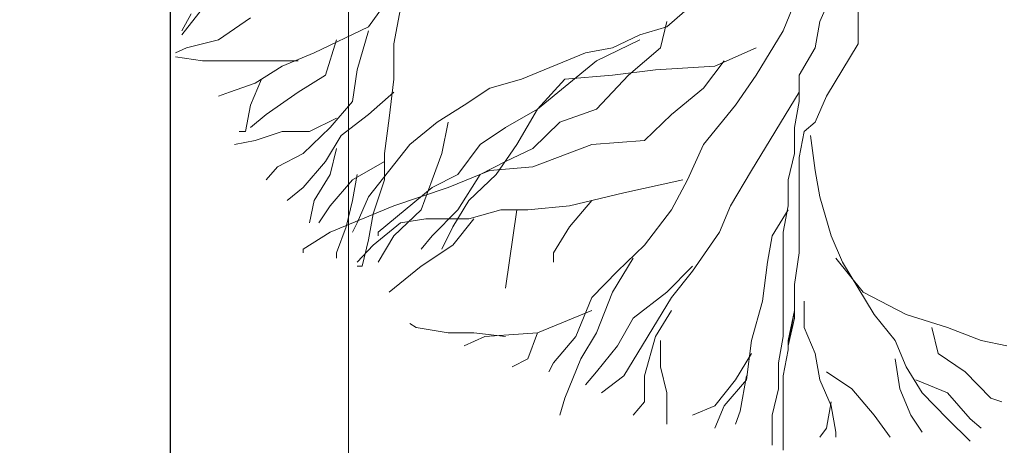
# Model space of a CAD drawing. Units: millimetres. Extents: x 595116 to 630915, y 909473 to 920225.
# Tile 15 of 134: x 629500 to 629534, y 919202 to 919216. Entities that reach past the tile are written whole.
import ezdxf

# ---------------------------------------------------------------- set-up
doc = ezdxf.new("R2010")
doc.units = ezdxf.units.MM
doc.layers.add('Dimension', color=3, linetype='Continuous', lineweight=18)
doc.layers.add('L-PLNT', color=85, linetype='Continuous', lineweight=13)
doc.styles.get("Standard").update_dxf_attribs({"font": 'arial.ttf'})
doc.dimstyles.new('ISO-25', dxfattribs={"dimtxt": 9, "dimasz": 6, "dimexe": 1.25, "dimexo": 0.625, "dimtad": 1, "dimlunit": 4, "dimtxsty": 'Standard', "dimcen": 2.5, "dimadec": 0, "dimazin": 0, "dimtfac": 1, "dimtmove": 0, "dimatfit": 3, "dimfxl": 1, "dimarcsym": 0})

# ---------------------------------------------------------------- blocks, each defined once
blk = doc.blocks.new('A$C143125F4')
for p, q in [((2.593, 1.7651), (2.593, 1.3932)), ((1.0011, 1.5724), (0.9136, 1.4515)), ((2.3906, 1.5724), (2.3359, 1.438)), ((2.4617, 1.4694), (2.5, 1.559)), ((2.0241, 1.5276), (1.9366, 1.4515)), ((0.2735, 1.4246), (0.3446, 1.5142)), ((0.3063, 1.4963), (0.2735, 1.438)), ((1.023, 1.5142), (1.0011, 1.3932)), ((0.5088, 1.4828), (0.3993, 1.4067)), ((1.9366, 1.4694), (1.9147, 1.3798)), ((2.4453, 1.3798), (2.4617, 1.4694)), ((0.9136, 1.4515), (0.7276, 1.3619)), ((0.9136, 1.438), (0.8753, 1.3036)), ((1.8436, 1.4246), (1.7506, 1.3798)), ((1.9366, 1.4515), (1.8436, 1.4246)), ((2.3359, 1.438), (2.2429, 1.2857)), ((0.3993, 1.4067), (0.2899, 1.3798)), ((0.8042, 1.4067), (0.7659, 1.2857)), ((1.0011, 1.3932), (1.0011, 1.2723)), ((1.8436, 1.4067), (1.6959, 1.335)), ((2.593, 1.3932), (2.4836, 1.214)), ((0.2899, 1.3798), (0.2516, 1.3619)), ((0.7276, 1.3619), (0.6182, 1.3171)), ((1.6576, 1.3619), (1.4387, 1.2723)), ((1.7506, 1.3798), (1.6576, 1.3619)), ((1.9147, 1.3798), (1.8053, 1.2857)), ((2.2429, 1.3798), (2.1007, 1.3171)), ((2.3906, 1.2857), (2.4453, 1.3798)), ((0.3446, 1.335), (0.2516, 1.3484)), ((0.6729, 1.335), (0.3446, 1.335)), ((0.6182, 1.3171), (0.5252, 1.2588)), ((1.6959, 1.335), (1.4935, 1.1692)), ((2.1007, 1.3171), (1.8983, 1.3036)), ((2.1335, 1.335), (2.0624, 1.2409)), ((0.7659, 1.2857), (0.6729, 1.2275)), ((0.8753, 1.3036), (0.8589, 1.1961)), ((1.7506, 1.2857), (1.5865, 1.2723)), ((1.8053, 1.2857), (1.6959, 1.1692)), ((1.8983, 1.3036), (1.7506, 1.2857)), ((2.2429, 1.2857), (2.1718, 1.1827)), ((2.3906, 1.1961), (2.3906, 1.2857)), ((0.5252, 1.2588), (0.4376, 1.2275)), ((0.5471, 1.2723), (0.5088, 1.1827)), ((1.0011, 1.2723), (0.9847, 1.1379)), ((1.4387, 1.2723), (1.3293, 1.2409)), ((1.5865, 1.2723), (1.4935, 1.1692)), ((0.4376, 1.2275), (0.3993, 1.214)), ((0.6729, 1.2275), (0.5635, 1.1513)), ((1.0011, 1.2275), (0.9136, 1.1513)), ((1.3293, 1.2409), (1.2418, 1.1827)), ((2.0624, 1.2409), (1.953, 1.1513)), ((2.3906, 1.2275), (2.2265, 0.9587)), ((0.5088, 1.1827), (0.4923, 1.0931)), ((0.8589, 1.1961), (0.7823, 1.1065)), ((1.2418, 1.1827), (1.1488, 1.1244)), ((2.1718, 1.1827), (2.0624, 1.0483)), ((2.3742, 1.1065), (2.3906, 1.1961)), ((2.4836, 1.214), (2.4453, 1.1244)), ((0.5635, 1.1513), (0.5088, 1.1065)), ((0.9136, 1.1513), (0.8206, 1.0796)), ((1.4935, 1.1692), (1.384, 1.1065)), ((1.4935, 1.1692), (1.4223, 1.0483)), ((1.6959, 1.1692), (1.57, 1.1244)), ((1.953, 1.1513), (1.86, 1.0617)), ((0.8042, 1.1379), (0.7112, 1.0931)), ((0.9847, 1.1379), (0.9683, 1.0169)), ((1.1488, 1.1244), (1.0558, 1.0483)), ((1.1871, 1.1244), (1.1652, 1.0169)), ((1.57, 1.1244), (1.477, 1.0348)), ((2.4453, 1.1244), (2.407, 1.0931)), ((0.4923, 1.0931), (0.4705, 1.0931)), ((0.6182, 1.0931), (0.5252, 1.0617)), ((0.7112, 1.0931), (0.6182, 1.0931)), ((0.7823, 1.1065), (0.6893, 1.0169)), ((1.384, 1.1065), (1.2965, 1.0483)), ((2.3742, 1.0169), (2.3742, 1.1065)), ((2.407, 1.0931), (2.3906, 1.0035)), ((0.5252, 1.0617), (0.4541, 1.0483)), ((0.8206, 1.0796), (0.7659, 0.99)), ((1.0558, 1.0483), (0.9136, 0.8691)), ((1.2965, 1.0483), (1.2199, 0.9452)), ((1.4223, 1.0483), (1.3512, 0.9452)), ((1.6795, 1.0483), (1.477, 0.9721)), ((1.86, 1.0617), (1.6795, 1.0483)), ((2.0624, 1.0483), (2.0077, 0.9273)), ((2.4289, 1.0796), (2.4453, 0.9587)), ((0.6893, 1.0169), (0.6018, 0.9721)), ((0.8042, 1.0348), (0.7823, 0.9452)), ((0.9683, 1.0169), (0.9683, 0.9273)), ((1.1652, 1.0169), (1.1324, 0.9273)), ((1.477, 1.0348), (1.384, 0.99)), ((2.3523, 0.9273), (2.3742, 1.0169)), ((0.7659, 0.99), (0.6893, 0.9005)), ((0.9683, 0.99), (0.8589, 0.9273)), ((1.384, 0.99), (1.2965, 0.9452)), ((2.3906, 1.0035), (2.3906, 0.6765)), ((0.6018, 0.9721), (0.5635, 0.9273)), ((0.7823, 0.9452), (0.7276, 0.8557)), ((0.8753, 0.9452), (0.8589, 0.8557)), ((1.2199, 0.9452), (1.1324, 0.9005)), ((1.3293, 0.9587), (1.1871, 0.9005)), ((1.2965, 0.9452), (1.2199, 0.8243)), ((1.3512, 0.9452), (1.2582, 0.8557)), ((1.477, 0.9721), (1.3293, 0.9587)), ((2.2265, 0.9587), (2.1554, 0.8377)), ((2.4453, 0.9587), (2.4617, 0.8691)), ((0.8589, 0.9273), (0.7823, 0.8377)), ((0.9683, 0.9273), (0.93, 0.8109)), ((1.1324, 0.9273), (1.0941, 0.8243)), ((1.9913, 0.9273), (1.7889, 0.8825)), ((2.0077, 0.9273), (1.953, 0.8243)), ((2.3523, 0.8377), (2.3523, 0.9273)), ((0.6893, 0.9005), (0.6346, 0.8557)), ((1.1324, 0.9005), (0.9464, 0.7481)), ((1.1871, 0.9005), (1.0011, 0.8377)), ((1.7889, 0.8825), (1.6029, 0.8377)), ((0.7276, 0.8557), (0.7112, 0.7795)), ((0.8589, 0.8557), (0.837, 0.7661)), ((0.9136, 0.8691), (0.8753, 0.7795)), ((1.2582, 0.8557), (1.2035, 0.7661)), ((1.6795, 0.8557), (1.6029, 0.7661)), ((2.4617, 0.8691), (2.5, 0.7347)), ((0.7823, 0.8377), (0.744, 0.7795)), ((1.0011, 0.8377), (0.7823, 0.7481)), ((0.93, 0.8109), (0.9136, 0.7213)), ((1.0941, 0.8243), (1.0011, 0.7347)), ((1.2199, 0.8243), (1.1324, 0.7347)), ((1.3676, 0.8243), (1.2582, 0.7929)), ((1.4606, 0.8243), (1.3676, 0.8243)), ((1.4223, 0.8243), (1.384, 0.5555)), ((1.6029, 0.8377), (1.4606, 0.8243)), ((1.953, 0.8243), (1.86, 0.7033)), ((2.1554, 0.8377), (2.1171, 0.7481)), ((2.3523, 0.8243), (2.2976, 0.7347)), ((2.3359, 0.7481), (2.3523, 0.8377)), ((0.8753, 0.7795), (0.8589, 0.7481)), ((1.023, 0.7795), (0.93, 0.7033)), ((1.1105, 0.7929), (1.023, 0.7795)), ((1.2582, 0.7929), (1.1105, 0.7929)), ((1.2746, 0.7929), (1.2035, 0.7033)), ((0.7823, 0.7481), (0.6893, 0.6899)), ((0.837, 0.7661), (0.8042, 0.6765)), ((0.9464, 0.7481), (0.9464, 0.7347)), ((1.2035, 0.7661), (1.1652, 0.6899)), ((1.6029, 0.7661), (1.5482, 0.6765)), ((2.1171, 0.7481), (2.0241, 0.6137)), ((2.3359, 0.3897), (2.3359, 0.7481)), ((0.9136, 0.7213), (0.8917, 0.6317)), ((1.0011, 0.7347), (0.9464, 0.6451)), ((1.1324, 0.7347), (1.0941, 0.6899)), ((2.2976, 0.7347), (2.2812, 0.6451)), ((2.5, 0.7347), (2.5383, 0.6451)), ((0.6893, 0.6899), (0.6893, 0.6765)), ((0.8042, 0.6765), (0.8042, 0.6585)), ((0.93, 0.7033), (0.8753, 0.6451)), ((1.2035, 0.7033), (1.0941, 0.6317)), ((1.5482, 0.6765), (1.5482, 0.6451)), ((1.86, 0.7033), (1.767, 0.6137)), ((2.3906, 0.6765), (2.3742, 0.5689)), ((1.8217, 0.6585), (1.7506, 0.5421)), ((2.2812, 0.6451), (2.2648, 0.5107)), ((2.5164, 0.6585), (2.6094, 0.5421)), ((2.5383, 0.6451), (2.6477, 0.4659)), ((0.8917, 0.6317), (0.8753, 0.6317)), ((1.0941, 0.6317), (0.9847, 0.5421)), ((1.767, 0.6137), (1.6795, 0.5241)), ((2.0241, 0.6317), (1.9366, 0.5421)), ((2.0241, 0.6137), (1.953, 0.5241)), ((1.7506, 0.5421), (1.6959, 0.4032)), ((1.9366, 0.5421), (1.8217, 0.4525)), ((2.3742, 0.5689), (2.3742, 0.4525)), ((2.6094, 0.5421), (2.7571, 0.4659)), ((1.6795, 0.5241), (1.6247, 0.3897)), ((1.953, 0.5241), (1.7889, 0.2554)), ((2.2648, 0.5107), (2.2265, 0.3763)), ((2.407, 0.5107), (2.407, 0.4211)), ((1.6795, 0.4793), (1.4935, 0.4032)), ((1.953, 0.4793), (1.8983, 0.3897)), ((2.3523, 0.3584), (2.3742, 0.4793)), ((2.3742, 0.4793), (2.3523, 0.3763)), ((1.8217, 0.4525), (1.767, 0.3584)), ((2.3742, 0.4525), (2.3523, 0.3584)), ((2.6477, 0.4659), (2.7189, 0.3763)), ((2.7571, 0.4659), (2.8994, 0.4211)), ((1.0777, 0.4211), (1.0558, 0.4345)), ((1.1871, 0.4032), (1.0777, 0.4211)), ((2.407, 0.4211), (2.4453, 0.3315)), ((2.8447, 0.4211), (2.8666, 0.3315)), ((2.8994, 0.4211), (3.0143, 0.3763)), ((1.2746, 0.4032), (1.1871, 0.4032)), ((1.3129, 0.3897), (1.2418, 0.3584)), ((1.384, 0.3897), (1.2746, 0.4032)), ((1.4935, 0.4032), (1.3129, 0.3897)), ((1.4935, 0.4032), (1.4606, 0.3136)), ((1.6247, 0.3897), (1.5482, 0.3002)), ((1.6959, 0.4032), (1.6412, 0.3136)), ((1.8983, 0.3897), (1.86, 0.2554)), ((1.9147, 0.3763), (1.9147, 0.2867)), ((2.2265, 0.3763), (2.2101, 0.2419)), ((2.3195, 0.3002), (2.3359, 0.3897)), ((2.3523, 0.3763), (2.3523, 0.3449)), ((2.7189, 0.3763), (2.7571, 0.2867)), ((3.0143, 0.3763), (3.1018, 0.3584)), ((1.767, 0.3584), (1.6959, 0.2688)), ((2.3523, 0.3449), (2.3359, 0.2554)), ((1.4606, 0.3136), (1.4059, 0.2867)), ((1.6412, 0.3136), (1.5865, 0.1792)), ((2.2265, 0.3315), (2.1718, 0.2419)), ((2.4453, 0.3315), (2.4617, 0.2419)), ((2.7189, 0.3136), (2.7353, 0.2106)), ((2.8666, 0.3315), (2.9596, 0.2688)), ((1.5482, 0.3002), (1.5317, 0.2688)), ((1.9147, 0.2867), (1.9366, 0.1971)), ((2.3195, 0.2106), (2.3195, 0.3002)), ((2.7571, 0.2867), (2.8119, 0.1971)), ((1.6959, 0.2688), (1.6576, 0.224)), ((1.7889, 0.2554), (1.7123, 0.1971)), ((1.86, 0.2554), (1.86, 0.1658)), ((2.1718, 0.2419), (2.1007, 0.1523)), ((2.2101, 0.2419), (2.1335, 0.1523)), ((2.2101, 0.2554), (2.1882, 0.1344)), ((2.3359, 0.2554), (2.3359, 0)), ((2.4617, 0.2419), (2.5, 0.1523)), ((2.4836, 0.2688), (2.5711, 0.2106)), ((2.79, 0.2419), (2.8994, 0.1971)), ((2.9596, 0.2688), (3.0471, 0.1792)), ((2.2976, 0.121), (2.3195, 0.2106)), ((2.5711, 0.2106), (2.6477, 0.121)), ((2.7353, 0.2106), (2.7736, 0.121)), ((1.5865, 0.1792), (1.57, 0.121)), ((1.9366, 0.1971), (1.9366, 0.0896)), ((2.8119, 0.1971), (2.8994, 0.1075)), ((2.8994, 0.1971), (2.976, 0.1075)), ((3.0471, 0.1792), (3.0854, 0.1658)), ((1.86, 0.1658), (1.8217, 0.121)), ((2.1007, 0.1523), (2.0241, 0.121)), ((2.1335, 0.1523), (2.1007, 0.0762)), ((2.5, 0.1658), (2.4836, 0.0762)), ((2.5, 0.1523), (2.5164, 0.0627)), ((2.1882, 0.1344), (2.1718, 0.0896)), ((2.2976, 0.0179), (2.2976, 0.121)), ((2.6477, 0.121), (2.7024, 0.0448)), ((2.7736, 0.121), (2.8119, 0.0627)), ((2.8994, 0.1075), (2.976, 0.0314)), ((2.976, 0.1075), (3.0143, 0.0762)), ((2.4836, 0.0762), (2.4617, 0.0448)), ((2.5164, 0.0627), (2.5164, 0.0448))]:
    blk.add_line(p, q)
blk = doc.blocks.new('*D215')
at = {"layer": 'Defpoints', "color": 0, "transparency": 16777216}
for p in [(629316.041, 919411.828), (629505.041, 919411.828), (629505.041, 918832.378)]:
    blk.add_point(p, dxfattribs=at)
at = {"layer": 'Dimension', "color": 0, "lineweight": -2, "transparency": 16777216}
for p, q in [((629316.041, 919411.203), (629316.041, 918831.128)), ((629505.041, 919411.203), (629505.041, 918831.128)), ((629322.041, 918832.378), (629499.041, 918832.378))]:
    blk.add_line(p, q, dxfattribs=at)
at = {"layer": 'Dimension', "color": 0, "transparency": 16777216}
for points in [[(629322.041, 918833.378), (629322.041, 918831.378), (629316.041, 918832.378)], [(629499.041, 918833.378), (629499.041, 918831.378), (629505.041, 918832.378)]]:
    blk.add_solid(points, dxfattribs=at)
at = {"layer": 'Dimension', "color": 0, "transparency": 16777216, "insert": (629410.541, 918837.598), "char_height": 9, "attachment_point": 5}
blk.add_mtext('15\'-9"', dxfattribs=at)
blk = doc.blocks.new('*D216')
at = {"layer": 'Defpoints', "color": 0, "transparency": 16777216}
for p in [(629505.041, 919411.828), (629743.541, 919411.928), (629743.541, 918832.378)]:
    blk.add_point(p, dxfattribs=at)
at = {"layer": 'Dimension', "color": 0, "lineweight": -2, "transparency": 16777216}
for p, q in [((629505.041, 919411.203), (629505.041, 918831.128)), ((629743.541, 919411.303), (629743.541, 918831.128)), ((629511.041, 918832.378), (629737.541, 918832.378))]:
    blk.add_line(p, q, dxfattribs=at)
at = {"layer": 'Dimension', "color": 0, "transparency": 16777216}
for points in [[(629511.041, 918833.378), (629511.041, 918831.378), (629505.041, 918832.378)], [(629737.541, 918833.378), (629737.541, 918831.378), (629743.541, 918832.378)]]:
    blk.add_solid(points, dxfattribs=at)
at = {"layer": 'Dimension', "color": 0, "transparency": 16777216, "insert": (629624.291, 918837.656), "char_height": 9, "attachment_point": 5}
blk.add_mtext('19\'-10 1/2"', dxfattribs=at)
blk = doc.blocks.new('*D221')
at = {"layer": 'Defpoints', "color": 0, "transparency": 16777216}
for p in [(629511.274, 919302.009), (629155.382, 919160.917), (629511.274, 919160.917)]:
    blk.add_point(p, dxfattribs=at)
at = {"layer": 'Dimension', "color": 0, "lineweight": -2, "transparency": 16777216}
for p, q in [((629510.649, 919302.009), (629154.132, 919302.009)), ((629155.382, 919296.009), (629155.382, 919166.917)), ((629510.649, 919160.917), (629154.132, 919160.917))]:
    blk.add_line(p, q, dxfattribs=at)
at = {"layer": 'Dimension', "color": 0, "transparency": 16777216}
for points in [[(629154.382, 919296.009), (629156.382, 919296.009), (629155.382, 919302.009)], [(629154.382, 919166.917), (629156.382, 919166.917), (629155.382, 919160.917)]]:
    blk.add_solid(points, dxfattribs=at)
at = {"layer": 'Dimension', "color": 0, "transparency": 16777216, "insert": (629150.162, 919231.463), "char_height": 9, "attachment_point": 5, "rotation": 90}
blk.add_mtext('11\'-9"', dxfattribs=at)

msp = doc.modelspace()

# ---------------------------------------------------------------- linework, layer by layer
at = {"layer": 'L-PLNT'}
msp.add_line((629511.274, 919302.009), (629511.274, 919160.917), dxfattribs=at)

# ---------------------------------------------------------------- block references
at = {"layer": 'L-PLNT', "xscale": 10.20167662382051, "yscale": 10.20167662382051, "zscale": 10.20167662382051}
msp.add_blockref('A$C143125F4', (629502.654, 919201.332), dxfattribs=at)

# ---------------------------------------------------------------- dimensions: what is measured, and where the dimension line sits
at = {"layer": 'Dimension'}
for base, p1, p2, picture, middle in [((629505.041, 918832.378), (629316.041, 919411.828), (629505.041, 919411.828), '*D215', (629410.541, 918837.598)), ((629743.541, 918832.378), (629505.041, 919411.828), (629743.541, 919411.928), '*D216', (629624.291, 918837.656))]:
    dim = msp.add_linear_dim(base=base, p1=p1, p2=p2, dimstyle='ISO-25', override={"dimdec": 1, "dimlfac": 1, "dimrnd": 0, "dimzin": 1, "dimdsep": 46, "dimlunit": 4, "dimfrac": 2}, dxfattribs=at)
    dim.commit()
    dim.dimension.update_dxf_attribs({"geometry": picture, "text_midpoint": middle})
dim = msp.add_linear_dim(base=(629155.382, 919160.917), p1=(629511.274, 919302.009), p2=(629511.274, 919160.917), angle=90, dimstyle='ISO-25', override={"dimdec": 1, "dimlfac": 1, "dimrnd": 0, "dimzin": 1, "dimdsep": 46, "dimlunit": 4, "dimfrac": 2}, dxfattribs=at)
dim.commit()
dim.dimension.update_dxf_attribs({"geometry": '*D221', "text_midpoint": (629150.162, 919231.463)})

doc.saveas('drawing.dxf')
